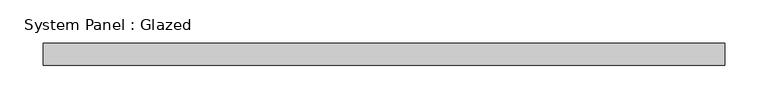
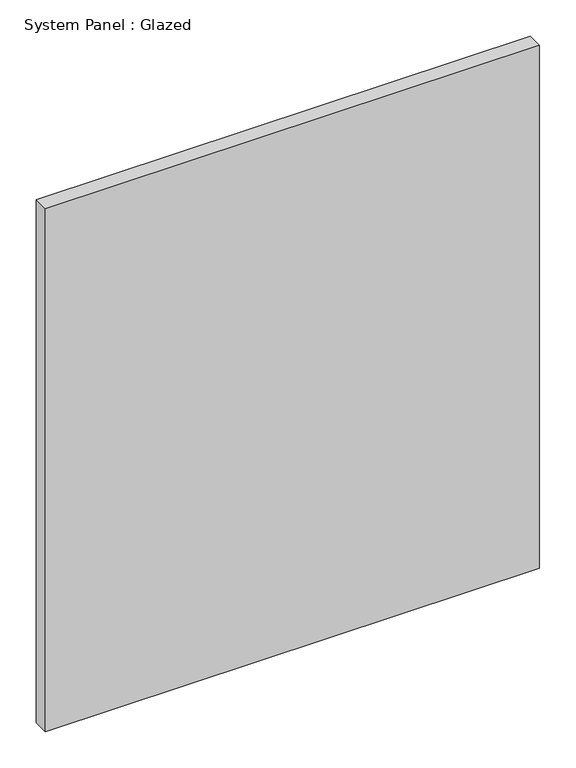
"""IFC4 building model written with IfcOpenShell, lengths in millimetres: plate geometry, System Panel : Glazed."""

from ifc_helpers import new_model, si_unit, origin, origin_with_axes, place, context, project, spatial, polyline, outline, extrude, source, transform, mapped, element, save


def system_panel_glazed_66480490(model_context):
    return source(origin(), model_context, "Body", "SweptSolid", [
        extrude(outline(polyline([(394.3296124, 19.05), (-394.3296124, 19.05), (-394.3296124, 44.45), (394.3296124, 44.45), (394.3296124, 19.05)])), origin_with_axes(), (0.0, 0.0, 1.0), 882.384107),
    ])


if __name__ == "__main__":
    model = new_model("IFC4")
    model_context = context("Model", 3, world=origin())
    ifc_project = project(units=[si_unit("LENGTHUNIT", "METRE", prefix="MILLI")], contexts=[model_context])
    site = spatial("IfcSite", under=ifc_project)
    building = spatial("IfcBuilding", under=site)
    placement = place(None, origin())
    system_panel_glazed_shape = system_panel_glazed_66480490(model_context)
    element("IfcPlate", 1, ObjectType="System Panel : Glazed", at=placement, inside=building, context=model_context, shape_type="MappedRepresentation", body=[
        mapped(system_panel_glazed_shape, transform((0.0, 0.0, 0.0), x_axis=(1.0, 0.0, 0.0), y_axis=(0.0, 1.0, 0.0), z_axis=(0.0, 0.0, 1.0))),
    ])
    save(model, "model.ifc")

# Revit data of these elements
# Type "System Panel : Glazed"
#   Construction Type Id = "GSP4R"
#   Analytic Construction = "1/8 in Pilkington single glazing"
#   Visual Light Transmittance = 0.9
#   Solar Heat Gain Coefficient = 0.86
#   Heat Transfer Coefficient (U) = 1.18115 BTU/(h·ft²·°F)
# Element 1 (IfcPlate, "System Panel : Glazed")
#   Materials on its faces: "Glass"
# Materials
#   "Glass": class "Glass", colour RGB 0 128 192, transparency 0.75, Description = "Soda Lime Glass", Cost = 0
